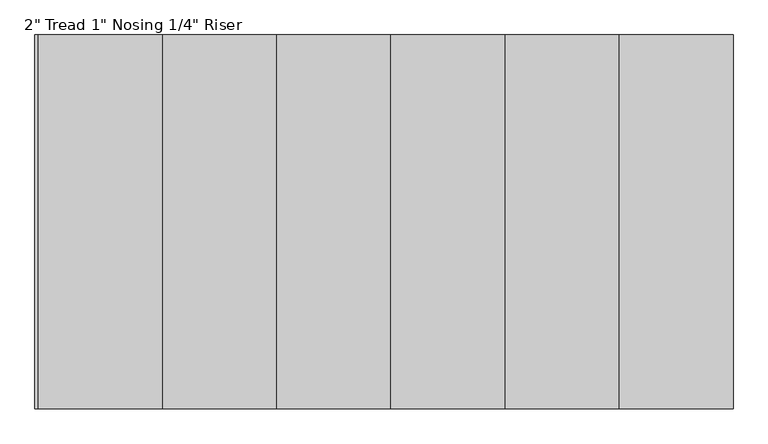
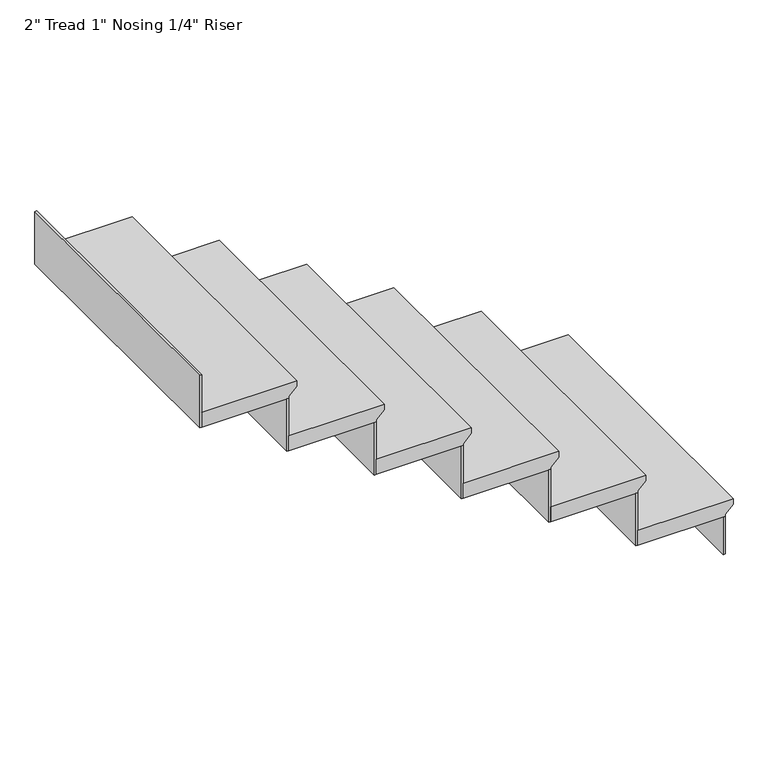
"""IFC4 building model written with IfcOpenShell, lengths in millimetres: stair flight geometry."""

from ifc_helpers import new_model, si_unit, origin, place, context, project, spatial, faceted_brep, source, transform, mapped, element, save


def stair_flight_c0af1c60(model_context):
    return source(origin(), model_context, "Body", "Brep", [
        faceted_brep([(-6576.0763529, -1051.6338022, 3968.75), (-6576.0763529, -1051.6338022, 3987.8), (-6576.0763529, -1966.0338022, 3987.8), (-6576.0763529, -1966.0338022, 3968.75), (-6601.4763529, -1051.6338022, 3943.35), (-6601.4763529, -1966.0338022, 3943.35), (-6880.8763529, -1051.6338022, 3987.8), (-6880.8763529, -1966.0338022, 3987.8), (-6601.4763529, -1966.0338022, 3937.0), (-6880.8763529, -1966.0338022, 3937.0), (-6880.8763529, -1051.6338022, 3937.0), (-6601.4763529, -1051.6338022, 3937.0)], [[[0, 1, 2, 3]], [[4, 0, 3, 5]], [[2, 1, 6, 7]], [[8, 9, 10, 11]], [[2, 7, 9, 8, 5, 3]], [[8, 11, 4, 5]], [[6, 1, 0, 4, 11, 10]], [[7, 6, 10, 9]]]),
        faceted_brep([(-6601.4763529, -1051.6338022, 3937.0), (-6601.4763529, -1051.6338022, 3810.0), (-6607.8263529, -1051.6338022, 3810.0), (-6607.8263529, -1051.6338022, 3937.0), (-6601.4763529, -1966.0338022, 3937.0), (-6607.8263529, -1966.0338022, 3937.0), (-6607.8263529, -1966.0338022, 3810.0), (-6601.4763529, -1966.0338022, 3810.0)], [[[0, 1, 2, 3]], [[4, 5, 6, 7]], [[1, 0, 4, 7]], [[2, 1, 7, 6]], [[3, 2, 6, 5]], [[0, 3, 5, 4]]]),
        faceted_brep([(-6880.8763529, -1051.6338022, 4114.8), (-6880.8763529, -1051.6338022, 3937.0), (-6887.2263529, -1051.6338022, 3937.0), (-6887.2263529, -1051.6338022, 4114.8), (-6880.8763529, -1966.0338022, 4114.8), (-6887.2263529, -1966.0338022, 4114.8), (-6887.2263529, -1966.0338022, 3937.0), (-6880.8763529, -1966.0338022, 3937.0)], [[[0, 1, 2, 3]], [[4, 5, 6, 7]], [[1, 0, 4, 7]], [[2, 1, 7, 6]], [[3, 2, 6, 5]], [[0, 3, 5, 4]]]),
        faceted_brep([(-6855.4763529, -1966.0338022, 4165.6), (-6855.4763529, -1051.6338022, 4165.6), (-7160.2763529, -1051.6338022, 4165.6), (-7160.2763529, -1966.0338022, 4165.6), (-6880.8763529, -1966.0338022, 4114.8), (-7160.2763529, -1966.0338022, 4114.8), (-7160.2763529, -1051.6338022, 4114.8), (-6880.8763529, -1051.6338022, 4114.8), (-6880.8763529, -1966.0338022, 4121.15), (-6855.4763529, -1966.0338022, 4146.55), (-6880.8763529, -1051.6338022, 4121.15), (-6855.4763529, -1051.6338022, 4146.55)], [[[0, 1, 2, 3]], [[4, 5, 6, 7]], [[0, 3, 5, 4, 8, 9]], [[4, 7, 10, 8]], [[2, 1, 11, 10, 7, 6]], [[3, 2, 6, 5]], [[11, 1, 0, 9]], [[10, 11, 9, 8]]]),
        faceted_brep([(-7160.2763529, -1051.6338022, 4292.6), (-7160.2763529, -1051.6338022, 4114.8), (-7166.6263529, -1051.6338022, 4114.8), (-7166.6263529, -1051.6338022, 4292.6), (-7160.2763529, -1966.0338022, 4292.6), (-7166.6263529, -1966.0338022, 4292.6), (-7166.6263529, -1966.0338022, 4114.8), (-7160.2763529, -1966.0338022, 4114.8)], [[[0, 1, 2, 3]], [[4, 5, 6, 7]], [[1, 0, 4, 7]], [[2, 1, 7, 6]], [[3, 2, 6, 5]], [[0, 3, 5, 4]]]),
        faceted_brep([(-7134.8763529, -1966.0338022, 4343.4), (-7134.8763529, -1051.6338022, 4343.4), (-7439.6763529, -1051.6338022, 4343.4), (-7439.6763529, -1966.0338022, 4343.4), (-7160.2763529, -1966.0338022, 4292.6), (-7439.6763529, -1966.0338022, 4292.6), (-7439.6763529, -1051.6338022, 4292.6), (-7160.2763529, -1051.6338022, 4292.6), (-7160.2763529, -1966.0338022, 4298.95), (-7134.8763529, -1966.0338022, 4324.35), (-7160.2763529, -1051.6338022, 4298.95), (-7134.8763529, -1051.6338022, 4324.35)], [[[0, 1, 2, 3]], [[4, 5, 6, 7]], [[0, 3, 5, 4, 8, 9]], [[4, 7, 10, 8]], [[2, 1, 11, 10, 7, 6]], [[3, 2, 6, 5]], [[11, 1, 0, 9]], [[10, 11, 9, 8]]]),
        faceted_brep([(-7439.6763529, -1051.6338022, 4470.4), (-7439.6763529, -1051.6338022, 4292.6), (-7446.0263529, -1051.6338022, 4292.6), (-7446.0263529, -1051.6338022, 4470.4), (-7439.6763529, -1966.0338022, 4470.4), (-7446.0263529, -1966.0338022, 4470.4), (-7446.0263529, -1966.0338022, 4292.6), (-7439.6763529, -1966.0338022, 4292.6)], [[[0, 1, 2, 3]], [[4, 5, 6, 7]], [[1, 0, 4, 7]], [[2, 1, 7, 6]], [[3, 2, 6, 5]], [[0, 3, 5, 4]]]),
        faceted_brep([(-7414.2763529, -1966.0338022, 4521.2), (-7414.2763529, -1051.6338022, 4521.2), (-7719.0763529, -1051.6338022, 4521.2), (-7719.0763529, -1966.0338022, 4521.2), (-7439.6763529, -1966.0338022, 4470.4), (-7719.0763529, -1966.0338022, 4470.4), (-7719.0763529, -1051.6338022, 4470.4), (-7439.6763529, -1051.6338022, 4470.4), (-7439.6763529, -1966.0338022, 4476.75), (-7414.2763529, -1966.0338022, 4502.15), (-7439.6763529, -1051.6338022, 4476.75), (-7414.2763529, -1051.6338022, 4502.15)], [[[0, 1, 2, 3]], [[4, 5, 6, 7]], [[0, 3, 5, 4, 8, 9]], [[4, 7, 10, 8]], [[2, 1, 11, 10, 7, 6]], [[3, 2, 6, 5]], [[11, 1, 0, 9]], [[10, 11, 9, 8]]]),
        faceted_brep([(-7719.0763529, -1051.6338022, 4648.2), (-7719.0763529, -1051.6338022, 4470.4), (-7725.4263529, -1051.6338022, 4470.4), (-7725.4263529, -1051.6338022, 4648.2), (-7719.0763529, -1966.0338022, 4648.2), (-7725.4263529, -1966.0338022, 4648.2), (-7725.4263529, -1966.0338022, 4470.4), (-7719.0763529, -1966.0338022, 4470.4)], [[[0, 1, 2, 3]], [[4, 5, 6, 7]], [[1, 0, 4, 7]], [[2, 1, 7, 6]], [[3, 2, 6, 5]], [[0, 3, 5, 4]]]),
        faceted_brep([(-7693.6763529, -1966.0338022, 4699.0), (-7693.6763529, -1051.6338022, 4699.0), (-7998.4763529, -1051.6338022, 4699.0), (-7998.4763529, -1966.0338022, 4699.0), (-7719.0763529, -1966.0338022, 4648.2), (-7998.4763529, -1966.0338022, 4648.2), (-7998.4763529, -1051.6338022, 4648.2), (-7719.0763529, -1051.6338022, 4648.2), (-7719.0763529, -1966.0338022, 4654.55), (-7693.6763529, -1966.0338022, 4679.95), (-7719.0763529, -1051.6338022, 4654.55), (-7693.6763529, -1051.6338022, 4679.95)], [[[0, 1, 2, 3]], [[4, 5, 6, 7]], [[0, 3, 5, 4, 8, 9]], [[4, 7, 10, 8]], [[2, 1, 11, 10, 7, 6]], [[3, 2, 6, 5]], [[11, 1, 0, 9]], [[10, 11, 9, 8]]]),
        faceted_brep([(-8277.8763529, -1051.6338022, 5003.8), (-8277.8763529, -1051.6338022, 4826.0), (-8284.2263529, -1051.6338022, 4826.0), (-8284.2263529, -1051.6338022, 5003.8), (-8277.8763529, -1966.0338022, 5003.8), (-8284.2263529, -1966.0338022, 5003.8), (-8284.2263529, -1966.0338022, 4826.0), (-8277.8763529, -1966.0338022, 4826.0)], [[[0, 1, 2, 3]], [[4, 5, 6, 7]], [[1, 0, 4, 7]], [[2, 1, 7, 6]], [[3, 2, 6, 5]], [[0, 3, 5, 4]]]),
        faceted_brep([(-7998.4763529, -1051.6338022, 4826.0), (-7998.4763529, -1051.6338022, 4648.2), (-8004.8263529, -1051.6338022, 4648.2), (-8004.8263529, -1051.6338022, 4826.0), (-7998.4763529, -1966.0338022, 4826.0), (-8004.8263529, -1966.0338022, 4826.0), (-8004.8263529, -1966.0338022, 4648.2), (-7998.4763529, -1966.0338022, 4648.2)], [[[0, 1, 2, 3]], [[4, 5, 6, 7]], [[1, 0, 4, 7]], [[2, 1, 7, 6]], [[3, 2, 6, 5]], [[0, 3, 5, 4]]]),
        faceted_brep([(-7973.0763529, -1966.0338022, 4876.8), (-7973.0763529, -1051.6338022, 4876.8), (-8252.4763529, -1051.6338022, 4876.8), (-8277.8763529, -1051.6338022, 4876.8), (-8277.8763529, -1966.0338022, 4876.8), (-7998.4763529, -1966.0338022, 4826.0), (-8277.8763529, -1966.0338022, 4826.0), (-8277.8763529, -1051.6338022, 4826.0), (-8252.4763529, -1051.6338022, 4826.0), (-7998.4763529, -1051.6338022, 4826.0), (-7998.4763529, -1966.0338022, 4832.35), (-7973.0763529, -1966.0338022, 4857.75), (-7998.4763529, -1051.6338022, 4832.35), (-7973.0763529, -1051.6338022, 4857.75)], [[[0, 1, 2, 3, 4]], [[5, 6, 7, 8, 9]], [[0, 4, 6, 5, 10, 11]], [[5, 9, 12, 10]], [[2, 1, 13, 12, 9, 8]], [[3, 2, 8, 7]], [[4, 3, 7, 6]], [[13, 1, 0, 11]], [[12, 13, 11, 10]]]),
    ])


if __name__ == "__main__":
    model = new_model("IFC4")
    model_context = context("Model", 3, world=origin())
    ifc_project = project(units=[si_unit("LENGTHUNIT", "METRE", prefix="MILLI")], contexts=[model_context])
    site = spatial("IfcSite", under=ifc_project)
    building = spatial("IfcBuilding", under=site)
    placement = place(None, origin())
    stair_flight_shape = stair_flight_c0af1c60(model_context)
    element("IfcStairFlight", 1, ObjectType="2\" Tread 1\" Nosing 1/4\" Riser", at=placement, inside=building, context=model_context, shape_type="MappedRepresentation", body=[
        mapped(stair_flight_shape, transform((0.0, 0.0, 0.0), x_axis=(1.0, 0.0, 0.0), y_axis=(0.0, 1.0, 0.0), z_axis=(0.0, 0.0, 1.0))),
    ])
    save(model, "model.ifc")
